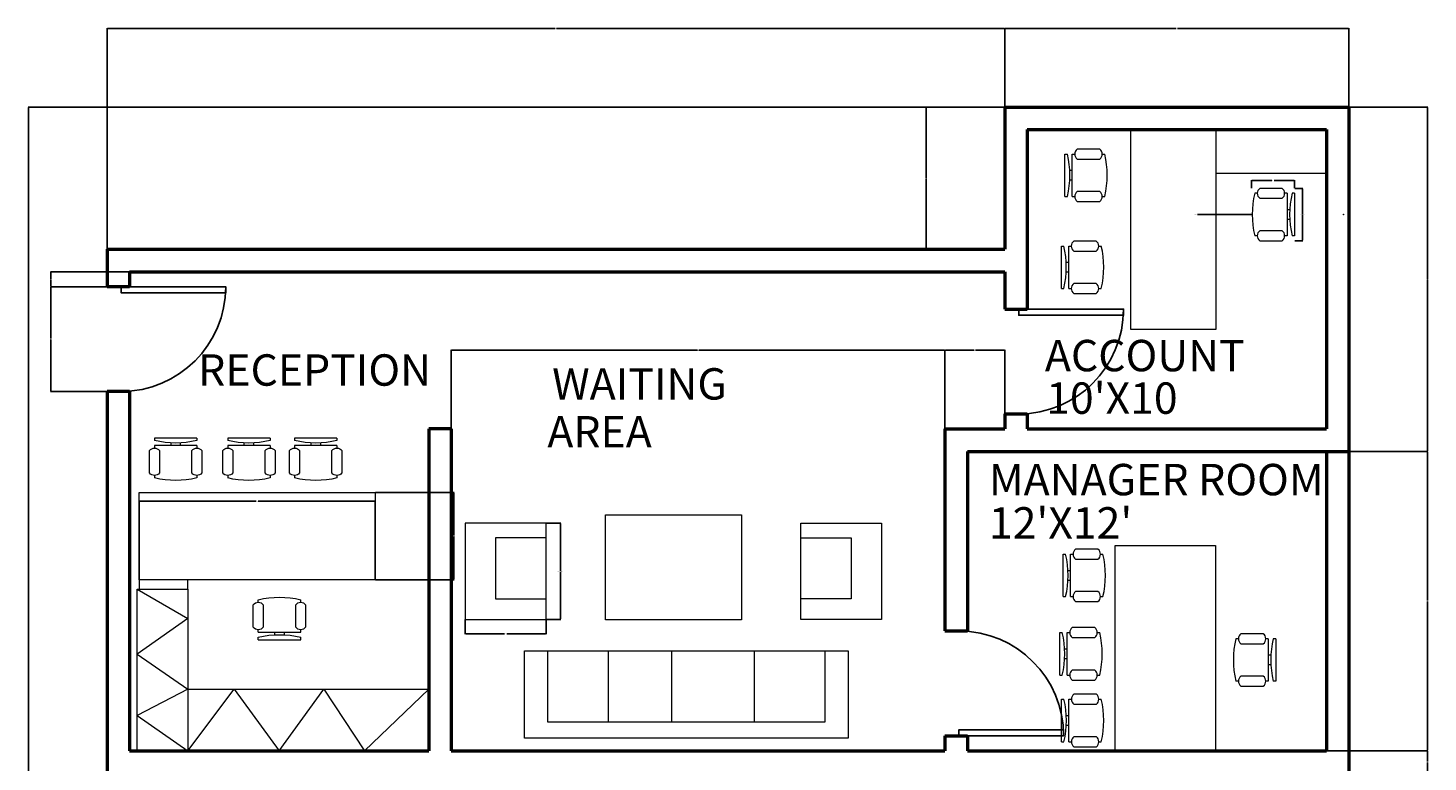
# Model space of a CAD drawing. Units: inches. Extents: x 4242 to 4803, y 4687 to 5377.
# Tile 2 of 2: x 4242 to 4803, y 5083 to 5377. Entities that reach past the tile are written whole.
import ezdxf

# ---------------------------------------------------------------- set-up
doc = ezdxf.new("R2010")
doc.units = ezdxf.units.IN
for name, color, linetype, lineweight in [('A-ANNO-DIMS', 2, 'Continuous', 18), ('A-AREA-IDEN', 7, 'Continuous', 25), ('A-DOOR', 4, 'Continuous', 25), ('A-FURN', 8, 'Continuous', 18), ('A-WALL', 7, 'Continuous', 50)]:
    doc.layers.add(name, color=color, linetype=linetype, lineweight=lineweight)
doc.styles.get("Standard").update_dxf_attribs({"font": 'arial.ttf'})
doc.dimstyles.get("Standard").update_dxf_attribs({"dimtxt": 0.18, "dimasz": 0.18, "dimexe": 0.18, "dimexo": 0.0625, "dimgap": 0.09, "dimtad": 0, "dimtih": 1, "dimtoh": 1, "dimdec": 4, "dimzin": 0, "dimdsep": 46, "dimtxsty": 'Standard', "dimcen": 0.09, "dimadec": 0, "dimazin": 0, "dimtfac": 1, "dimtdec": 4, "dimtofl": 0, "dimtmove": 0, "dimatfit": 3, "dimfxl": 1, "dimtolj": 1, "dimtzin": 0, "dimarcsym": 0})

# ---------------------------------------------------------------- blocks, each defined once
blk = doc.blocks.new('Chair - Desk')
for p, q in [((-8.5, 0), (-8.5, -1)), ((-8.5, 0), (8.5, 0)), ((8.5, 0), (8.5, -1)), ((-10.5, -5), (-10.5, -14)), ((-8.5, -3), (-8.5, -4)), ((-8.5, -3), (8.5, -3)), ((-6.5, -14), (-6.5, -5)), ((-2, -3), (-2, -1.9355)), ((2, -1.9576), (2, -3)), ((6.5, -5), (6.5, -14)), ((8.5, -3), (8.5, -4)), ((10.5, -14), (10.5, -5)), ((-8.5, -15), (-8.5, -16)), ((8.5, -15), (8.5, -16))]:
    blk.add_line(p, q)
for centre, radius, start, end in [((-8.5, -6.5), 2.5, 36.8699, 143.1301), ((0, 34.625), 36.625, 256.5803, 283.4197), ((8.5, -6.5), 2.5, 36.8699, 143.1301), ((-8.5, -12.5), 2.5, 216.8699, 323.1301), ((0, 19.625), 36.625, 256.5803, 283.4197), ((8.5, -12.5), 2.5, 216.8699, 323.1301)]:
    blk.add_arc(centre, radius, start, end)
blk = doc.blocks.new('*U4')
for p, q in [((0, 0), (0, -100)), ((750, 0), (750, -100))]:
    blk.add_line(p, q)
blk.add_lwpolyline([(0, 0), (0, 750), (43.75, 750), (43.75, 0)], close=True)
blk.add_arc((0, 0), 750, 0, 90)
blk = doc.blocks.new('CHAIR-LOUNGE')
for points in [[(32.4, 38.56), (0, 38.56), (0, 0), (32.4, 0)], [(32.4, 32.69), (12.18, 32.69), (12.18, 8.21), (32.4, 8.21)]]:
    blk.add_lwpolyline(points, close=True)
blk = doc.blocks.new('*D6')
at = {"layer": 'A-ANNO-DIMS', "color": 0, "lineweight": -2, "transparency": 16777216}
for p, q in [((4749.57, 5313.06), (4752.84, 5313.06)), ((4752.66, 5312.88), (4752.66, 5302.75)), ((4752.66, 5292.24), (4752.66, 5302.38)), ((4749.57, 5292.06), (4752.84, 5292.06))]:
    blk.add_line(p, q, dxfattribs=at)
at = {"layer": 'A-ANNO-DIMS', "color": 0, "transparency": 16777216}
for points in [[(4752.63, 5312.88), (4752.69, 5312.88), (4752.66, 5313.06)], [(4752.63, 5292.24), (4752.69, 5292.24), (4752.66, 5292.06)]]:
    blk.add_solid(points, dxfattribs=at)
at = {"layer": 'Defpoints', "color": 0, "transparency": 16777216}
for p in [(4749.51, 5313.06), (4749.51, 5292.06), (4752.66, 5292.06)]:
    blk.add_point(p, dxfattribs=at)
at = {"layer": 'A-ANNO-DIMS', "color": 0, "transparency": 16777216, "insert": (4752.66, 5302.56), "char_height": 0.18, "attachment_point": 5}
blk.add_mtext('\\A1;DESK CHAIR 21 TYP.', dxfattribs=at)
blk = doc.blocks.new('*D7')
at = {"layer": 'A-ANNO-DIMS', "color": 0, "lineweight": -2, "transparency": 16777216}
for p, q in [((4732.18, 5313.13), (4732.18, 5316.39)), ((4732.36, 5316.21), (4740.32, 5316.21)), ((4749.33, 5316.21), (4741.36, 5316.21)), ((4749.51, 5313.13), (4749.51, 5316.39))]:
    blk.add_line(p, q, dxfattribs=at)
at = {"layer": 'A-ANNO-DIMS', "color": 0, "transparency": 16777216}
for points in [[(4732.36, 5316.24), (4732.36, 5316.18), (4732.18, 5316.21)], [(4749.33, 5316.24), (4749.33, 5316.18), (4749.51, 5316.21)]]:
    blk.add_solid(points, dxfattribs=at)
at = {"layer": 'Defpoints', "color": 0, "transparency": 16777216}
for p in [(4732.18, 5313.06), (4749.51, 5316.21), (4749.51, 5313.06)]:
    blk.add_point(p, dxfattribs=at)
at = {"layer": 'A-ANNO-DIMS', "color": 0, "transparency": 16777216, "insert": (4740.84, 5316.21), "char_height": 0.18, "attachment_point": 5}
blk.add_mtext('\\A1;17 TYP.', dxfattribs=at)
blk = doc.blocks.new('*D10')
at = {"layer": 'A-ANNO-DIMS', "color": 0, "lineweight": -2, "transparency": 16777216}
for p, q in [((4449.39, 5178.86), (4455.29, 5178.86)), ((4455.11, 5178.68), (4455.11, 5159.77)), ((4455.11, 5140.48), (4455.11, 5159.4)), ((4449.39, 5140.3), (4455.29, 5140.3))]:
    blk.add_line(p, q, dxfattribs=at)
at = {"layer": 'A-ANNO-DIMS', "color": 0, "transparency": 16777216}
for points in [[(4455.08, 5178.68), (4455.14, 5178.68), (4455.11, 5178.86)], [(4455.08, 5140.48), (4455.14, 5140.48), (4455.11, 5140.3)]]:
    blk.add_solid(points, dxfattribs=at)
at = {"layer": 'Defpoints', "color": 0, "transparency": 16777216}
for p in [(4449.33, 5178.86), (4455.11, 5178.86), (4449.33, 5140.3)]:
    blk.add_point(p, dxfattribs=at)
at = {"layer": 'A-ANNO-DIMS', "color": 0, "transparency": 16777216, "insert": (4455.11, 5159.58), "char_height": 0.18, "attachment_point": 5}
blk.add_mtext('\\A1;LOUNGE CHAIR 39 TYP.', dxfattribs=at)
blk = doc.blocks.new('*D11')
at = {"layer": 'A-ANNO-DIMS', "color": 0, "lineweight": -2, "transparency": 16777216}
for p, q in [((4416.93, 5140.24), (4416.93, 5134.34)), ((4449.33, 5140.24), (4449.33, 5134.34)), ((4417.11, 5134.52), (4432.6, 5134.52)), ((4449.15, 5134.52), (4433.65, 5134.52))]:
    blk.add_line(p, q, dxfattribs=at)
at = {"layer": 'A-ANNO-DIMS', "color": 0, "transparency": 16777216}
for points in [[(4417.11, 5134.55), (4417.11, 5134.49), (4416.93, 5134.52)], [(4449.15, 5134.55), (4449.15, 5134.49), (4449.33, 5134.52)]]:
    blk.add_solid(points, dxfattribs=at)
at = {"layer": 'Defpoints', "color": 0, "transparency": 16777216}
for p in [(4416.93, 5140.3), (4449.33, 5140.3), (4449.33, 5134.52)]:
    blk.add_point(p, dxfattribs=at)
at = {"layer": 'A-ANNO-DIMS', "color": 0, "transparency": 16777216, "insert": (4433.13, 5134.52), "char_height": 0.18, "attachment_point": 5}
blk.add_mtext('\\A1;32 TYP.', dxfattribs=at)
blk = doc.blocks.new('*D13')
at = {"layer": 'A-ANNO-DIMS', "color": 0, "lineweight": -2, "transparency": 16777216}
for p, q in [((4633.22, 5345.64), (4241.6, 5345.64)), ((4241.78, 5345.46), (4241.78, 5032.32)), ((4241.78, 4718.82), (4241.78, 5031.96)), ((4273.22, 4718.64), (4241.6, 4718.64))]:
    blk.add_line(p, q, dxfattribs=at)
at = {"layer": 'A-ANNO-DIMS', "color": 0, "transparency": 16777216}
for points in [[(4241.75, 5345.46), (4241.81, 5345.46), (4241.78, 5345.64)], [(4241.75, 4718.82), (4241.81, 4718.82), (4241.78, 4718.64)]]:
    blk.add_solid(points, dxfattribs=at)
at = {"layer": 'Defpoints', "color": 0, "transparency": 16777216}
for p in [(4241.78, 5345.64), (4633.28, 5345.64), (4273.28, 4718.64)]:
    blk.add_point(p, dxfattribs=at)
at = {"layer": 'A-ANNO-DIMS', "color": 0, "transparency": 16777216, "insert": (4241.78, 5032.14), "char_height": 0.18, "attachment_point": 5}
blk.add_mtext('\\A1;627', dxfattribs=at)
blk = doc.blocks.new('*D14')
at = {"layer": 'A-ANNO-DIMS', "color": 0, "lineweight": -2, "transparency": 16777216}
for p, q in [((4273.28, 5288.7), (4273.28, 5377.32)), ((4273.46, 5377.14), (4453, 5377.14)), ((4633.1, 5377.14), (4453.57, 5377.14)), ((4633.28, 5288.7), (4633.28, 5377.32))]:
    blk.add_line(p, q, dxfattribs=at)
at = {"layer": 'A-ANNO-DIMS', "color": 0, "transparency": 16777216}
for points in [[(4273.46, 5377.17), (4273.46, 5377.11), (4273.28, 5377.14)], [(4633.1, 5377.17), (4633.1, 5377.11), (4633.28, 5377.14)]]:
    blk.add_solid(points, dxfattribs=at)
at = {"layer": 'Defpoints', "color": 0, "transparency": 16777216}
for p in [(4633.28, 5377.14), (4273.28, 5288.64), (4633.28, 5288.64)]:
    blk.add_point(p, dxfattribs=at)
at = {"layer": 'A-ANNO-DIMS', "color": 0, "transparency": 16777216, "insert": (4453.28, 5377.14), "char_height": 0.18, "attachment_point": 5}
blk.add_mtext('\\A1;360', dxfattribs=at)
blk = doc.blocks.new('*D15')
at = {"layer": 'A-ANNO-DIMS', "color": 0, "lineweight": -2, "transparency": 16777216}
for p, q in [((4633.28, 5345.7), (4633.28, 5377.32)), ((4633.46, 5377.14), (4702, 5377.14)), ((4771.1, 5377.14), (4702.56, 5377.14)), ((4771.28, 5345.7), (4771.28, 5377.32))]:
    blk.add_line(p, q, dxfattribs=at)
at = {"layer": 'A-ANNO-DIMS', "color": 0, "transparency": 16777216}
for points in [[(4633.46, 5377.17), (4633.46, 5377.11), (4633.28, 5377.14)], [(4771.1, 5377.17), (4771.1, 5377.11), (4771.28, 5377.14)]]:
    blk.add_solid(points, dxfattribs=at)
at = {"layer": 'Defpoints', "color": 0, "transparency": 16777216}
for p in [(4771.28, 5377.14), (4633.28, 5345.64), (4771.28, 5345.64)]:
    blk.add_point(p, dxfattribs=at)
at = {"layer": 'A-ANNO-DIMS', "color": 0, "transparency": 16777216, "insert": (4702.28, 5377.14), "char_height": 0.18, "attachment_point": 5}
blk.add_mtext('\\A1;138', dxfattribs=at)
blk = doc.blocks.new('*D21')
at = {"layer": 'A-ANNO-DIMS', "color": 0, "lineweight": -2, "transparency": 16777216}
for p, q in [((4762.35, 5087.64), (4802.96, 5087.64)), ((4802.78, 5087.46), (4802.78, 5083.32)), ((4802.78, 5078.82), (4802.78, 5082.96)), ((4762.35, 5078.64), (4802.96, 5078.64))]:
    blk.add_line(p, q, dxfattribs=at)
at = {"layer": 'A-ANNO-DIMS', "color": 0, "transparency": 16777216}
for points in [[(4802.75, 5087.46), (4802.81, 5087.46), (4802.78, 5087.64)], [(4802.75, 5078.82), (4802.81, 5078.82), (4802.78, 5078.64)]]:
    blk.add_solid(points, dxfattribs=at)
at = {"layer": 'Defpoints', "color": 0, "transparency": 16777216}
for p in [(4762.28, 5087.64), (4802.78, 5087.64), (4762.28, 5078.64)]:
    blk.add_point(p, dxfattribs=at)
at = {"layer": 'A-ANNO-DIMS', "color": 0, "transparency": 16777216, "insert": (4802.78, 5083.14), "char_height": 0.18, "attachment_point": 5}
blk.add_mtext('\\A1;9', dxfattribs=at)
blk = doc.blocks.new('*D22')
at = {"layer": 'A-ANNO-DIMS', "color": 0, "lineweight": -2, "transparency": 16777216}
for p, q in [((4762.35, 5207.64), (4802.96, 5207.64)), ((4802.78, 5207.46), (4802.78, 5147.82)), ((4802.78, 5087.82), (4802.78, 5147.46)), ((4762.35, 5087.64), (4802.96, 5087.64))]:
    blk.add_line(p, q, dxfattribs=at)
at = {"layer": 'A-ANNO-DIMS', "color": 0, "transparency": 16777216}
for points in [[(4802.75, 5207.46), (4802.81, 5207.46), (4802.78, 5207.64)], [(4802.75, 5087.82), (4802.81, 5087.82), (4802.78, 5087.64)]]:
    blk.add_solid(points, dxfattribs=at)
at = {"layer": 'Defpoints', "color": 0, "transparency": 16777216}
for p in [(4762.28, 5207.64), (4802.78, 5207.64), (4762.28, 5087.64)]:
    blk.add_point(p, dxfattribs=at)
at = {"layer": 'A-ANNO-DIMS', "color": 0, "transparency": 16777216, "insert": (4802.78, 5147.64), "char_height": 0.18, "attachment_point": 5}
blk.add_mtext('\\A1;120', dxfattribs=at)
blk = doc.blocks.new('*D23')
at = {"layer": 'A-ANNO-DIMS', "color": 0, "lineweight": -2, "transparency": 16777216}
for p, q in [((4771.35, 5345.64), (4802.96, 5345.64)), ((4802.78, 5345.46), (4802.78, 5276.82)), ((4802.78, 5207.82), (4802.78, 5276.46)), ((4762.35, 5207.64), (4802.96, 5207.64))]:
    blk.add_line(p, q, dxfattribs=at)
at = {"layer": 'A-ANNO-DIMS', "color": 0, "transparency": 16777216}
for points in [[(4802.75, 5345.46), (4802.81, 5345.46), (4802.78, 5345.64)], [(4802.75, 5207.82), (4802.81, 5207.82), (4802.78, 5207.64)]]:
    blk.add_solid(points, dxfattribs=at)
at = {"layer": 'Defpoints', "color": 0, "transparency": 16777216}
for p in [(4771.28, 5345.64), (4802.78, 5345.64), (4762.28, 5207.64)]:
    blk.add_point(p, dxfattribs=at)
at = {"layer": 'A-ANNO-DIMS', "color": 0, "transparency": 16777216, "insert": (4802.78, 5276.64), "char_height": 0.18, "attachment_point": 5}
blk.add_mtext('\\A1;138', dxfattribs=at)
blk = doc.blocks.new('*D24')
at = {"layer": 'A-ANNO-DIMS', "color": 0, "lineweight": -2, "transparency": 16777216}
for p, q in [((4633.22, 5345.64), (4601.6, 5345.64)), ((4601.78, 5345.46), (4601.78, 5317.32)), ((4601.78, 5288.82), (4601.78, 5316.96)), ((4633.22, 5288.64), (4601.6, 5288.64))]:
    blk.add_line(p, q, dxfattribs=at)
at = {"layer": 'A-ANNO-DIMS', "color": 0, "transparency": 16777216}
for points in [[(4601.75, 5345.46), (4601.81, 5345.46), (4601.78, 5345.64)], [(4601.75, 5288.82), (4601.81, 5288.82), (4601.78, 5288.64)]]:
    blk.add_solid(points, dxfattribs=at)
at = {"layer": 'Defpoints', "color": 0, "transparency": 16777216}
for p in [(4601.78, 5345.64), (4633.28, 5345.64), (4633.28, 5288.64)]:
    blk.add_point(p, dxfattribs=at)
at = {"layer": 'A-ANNO-DIMS', "color": 0, "transparency": 16777216, "insert": (4601.78, 5317.14), "char_height": 0.18, "attachment_point": 5}
blk.add_mtext('\\A1;57', dxfattribs=at)
blk = doc.blocks.new('*D26')
at = {"layer": 'A-ANNO-DIMS', "color": 0, "lineweight": -2, "transparency": 16777216}
for p, q in [((4282.22, 5273.64), (4250.6, 5273.64)), ((4250.78, 5273.46), (4250.78, 5252.82)), ((4250.78, 5231.82), (4250.78, 5252.46)), ((4282.22, 5231.64), (4250.6, 5231.64))]:
    blk.add_line(p, q, dxfattribs=at)
at = {"layer": 'A-ANNO-DIMS', "color": 0, "transparency": 16777216}
for points in [[(4250.75, 5273.46), (4250.81, 5273.46), (4250.78, 5273.64)], [(4250.75, 5231.82), (4250.81, 5231.82), (4250.78, 5231.64)]]:
    blk.add_solid(points, dxfattribs=at)
at = {"layer": 'Defpoints', "color": 0, "transparency": 16777216}
for p in [(4250.78, 5273.64), (4282.28, 5273.64), (4282.28, 5231.64)]:
    blk.add_point(p, dxfattribs=at)
at = {"layer": 'A-ANNO-DIMS', "color": 0, "transparency": 16777216, "insert": (4250.78, 5252.64), "char_height": 0.18, "attachment_point": 5}
blk.add_mtext('\\A1;42', dxfattribs=at)
blk = doc.blocks.new('*D27')
at = {"layer": 'A-ANNO-DIMS', "color": 0, "lineweight": -2, "transparency": 16777216}
for p, q in [((4282.22, 5279.64), (4250.6, 5279.64)), ((4250.78, 5279.46), (4250.78, 5276.82)), ((4282.22, 5273.64), (4250.6, 5273.64)), ((4250.78, 5273.82), (4250.78, 5276.46))]:
    blk.add_line(p, q, dxfattribs=at)
at = {"layer": 'A-ANNO-DIMS', "color": 0, "transparency": 16777216}
for points in [[(4250.75, 5279.46), (4250.81, 5279.46), (4250.78, 5279.64)], [(4250.75, 5273.82), (4250.81, 5273.82), (4250.78, 5273.64)]]:
    blk.add_solid(points, dxfattribs=at)
at = {"layer": 'Defpoints', "color": 0, "transparency": 16777216}
for p in [(4250.78, 5279.64), (4282.28, 5279.64), (4282.28, 5273.64)]:
    blk.add_point(p, dxfattribs=at)
at = {"layer": 'A-ANNO-DIMS', "color": 0, "transparency": 16777216, "insert": (4250.78, 5276.64), "char_height": 0.18, "attachment_point": 5}
blk.add_mtext('\\A1;6', dxfattribs=at)
blk = doc.blocks.new('*D30')
at = {"layer": 'A-ANNO-DIMS', "color": 0, "lineweight": -2, "transparency": 16777216}
for p, q in [((4411.28, 5216.7), (4411.28, 5248.32)), ((4411.46, 5248.14), (4510, 5248.14)), ((4609.1, 5248.14), (4510.56, 5248.14)), ((4609.28, 5216.7), (4609.28, 5248.32))]:
    blk.add_line(p, q, dxfattribs=at)
at = {"layer": 'A-ANNO-DIMS', "color": 0, "transparency": 16777216}
for points in [[(4411.46, 5248.17), (4411.46, 5248.11), (4411.28, 5248.14)], [(4609.1, 5248.17), (4609.1, 5248.11), (4609.28, 5248.14)]]:
    blk.add_solid(points, dxfattribs=at)
at = {"layer": 'Defpoints', "color": 0, "transparency": 16777216}
for p in [(4609.28, 5248.14), (4411.28, 5216.64), (4609.28, 5216.64)]:
    blk.add_point(p, dxfattribs=at)
at = {"layer": 'A-ANNO-DIMS', "color": 0, "transparency": 16777216, "insert": (4510.28, 5248.14), "char_height": 0.18, "attachment_point": 5}
blk.add_mtext('\\A1;198', dxfattribs=at)
blk = doc.blocks.new('*D31')
at = {"layer": 'A-ANNO-DIMS', "color": 0, "lineweight": -2, "transparency": 16777216}
for p, q in [((4609.28, 5216.7), (4609.28, 5248.32)), ((4609.46, 5248.14), (4621.06, 5248.14)), ((4633.1, 5248.14), (4621.5, 5248.14)), ((4633.28, 5216.7), (4633.28, 5248.32))]:
    blk.add_line(p, q, dxfattribs=at)
at = {"layer": 'A-ANNO-DIMS', "color": 0, "transparency": 16777216}
for points in [[(4609.46, 5248.17), (4609.46, 5248.11), (4609.28, 5248.14)], [(4633.1, 5248.17), (4633.1, 5248.11), (4633.28, 5248.14)]]:
    blk.add_solid(points, dxfattribs=at)
at = {"layer": 'Defpoints', "color": 0, "transparency": 16777216}
for p in [(4633.28, 5248.14), (4609.28, 5216.64), (4633.28, 5216.64)]:
    blk.add_point(p, dxfattribs=at)
at = {"layer": 'A-ANNO-DIMS', "color": 0, "transparency": 16777216, "insert": (4621.28, 5248.14), "char_height": 0.18, "attachment_point": 5}
blk.add_mtext('\\A1;24', dxfattribs=at)
blk = doc.blocks.new('*D37')
at = {"layer": 'A-ANNO-DIMS', "color": 0, "lineweight": -2, "transparency": 16777216}
for p, q in [((4286.13, 5156.26), (4286.13, 5187.88)), ((4286.31, 5187.7), (4333.08, 5187.7)), ((4380.64, 5187.7), (4333.87, 5187.7)), ((4380.82, 5156.26), (4380.82, 5187.88))]:
    blk.add_line(p, q, dxfattribs=at)
at = {"layer": 'A-ANNO-DIMS', "color": 0, "transparency": 16777216}
for points in [[(4286.31, 5187.73), (4286.31, 5187.67), (4286.13, 5187.7)], [(4380.64, 5187.73), (4380.64, 5187.67), (4380.82, 5187.7)]]:
    blk.add_solid(points, dxfattribs=at)
at = {"layer": 'Defpoints', "color": 0, "transparency": 16777216}
for p in [(4380.82, 5187.7), (4286.13, 5156.2), (4380.82, 5156.2)]:
    blk.add_point(p, dxfattribs=at)
at = {"layer": 'A-ANNO-DIMS', "color": 0, "transparency": 16777216, "insert": (4333.47, 5187.7), "char_height": 0.18, "attachment_point": 5}
blk.add_mtext('\\A1;94.69', dxfattribs=at)
blk = doc.blocks.new('*D38')
at = {"layer": 'A-ANNO-DIMS', "color": 0, "lineweight": -2, "transparency": 16777216}
for p, q in [((4380.88, 5191.18), (4412.5, 5191.18)), ((4412.32, 5191), (4412.32, 5173.87)), ((4412.32, 5156.38), (4412.32, 5173.51)), ((4380.88, 5156.2), (4412.5, 5156.2))]:
    blk.add_line(p, q, dxfattribs=at)
at = {"layer": 'A-ANNO-DIMS', "color": 0, "transparency": 16777216}
for points in [[(4412.29, 5191), (4412.35, 5191), (4412.32, 5191.18)], [(4412.29, 5156.38), (4412.35, 5156.38), (4412.32, 5156.2)]]:
    blk.add_solid(points, dxfattribs=at)
at = {"layer": 'Defpoints', "color": 0, "transparency": 16777216}
for p in [(4380.82, 5191.18), (4380.82, 5156.2), (4412.32, 5156.2)]:
    blk.add_point(p, dxfattribs=at)
at = {"layer": 'A-ANNO-DIMS', "color": 0, "transparency": 16777216, "insert": (4412.32, 5173.69), "char_height": 0.18, "attachment_point": 5}
blk.add_mtext('\\A1;34.98', dxfattribs=at)
blk = doc.blocks.new('*D41')
at = {"layer": 'A-ANNO-DIMS', "color": 0, "lineweight": -2, "transparency": 16777216}
for p, q in [((4710.54, 5302.56), (4732.33, 5302.56)), ((4769.05, 5302.56), (4769.23, 5302.56)), ((4769.14, 5302.47), (4769.14, 5302.65))]:
    blk.add_line(p, q, dxfattribs=at)
at = {"layer": 'A-ANNO-DIMS', "color": 0, "transparency": 16777216}
blk.add_solid([(4732.33, 5302.59), (4732.33, 5302.53), (4732.51, 5302.56)], dxfattribs=at)
at = {"layer": 'Defpoints', "color": 0, "transparency": 16777216}
for p in [(4732.51, 5302.56), (4769.14, 5302.56)]:
    blk.add_point(p, dxfattribs=at)
at = {"layer": 'A-ANNO-DIMS', "color": 0, "transparency": 16777216, "insert": (4709.72, 5302.56), "char_height": 0.18, "attachment_point": 5}
blk.add_mtext('\\A1;25X R36.625', dxfattribs=at)

msp = doc.modelspace()

# ---------------------------------------------------------------- linework, layer by layer
at = {"layer": 'A-FURN'}
for p, q in [((4305.7309, 5156.1997), (4286.1298, 5156.1997)), ((4286.1298, 5156.1997), (4286.1298, 5152.4595)), ((4305.7309, 5152.4595), (4305.7309, 5156.1997)), ((4285.3425, 5152.4595), (4305.7309, 5140.6038)), ((4305.7309, 5140.6038), (4285.3425, 5126.3034)), ((4285.3425, 5126.3034), (4305.7309, 5112.3436)), ((4474.2273, 5127.7417), (4474.2273, 5099.1557)), ((4499.6923, 5127.7417), (4499.6923, 5099.1557)), ((4532.7665, 5127.7417), (4532.7665, 5099.1557)), ((4305.7309, 5112.3436), (4285.3425, 5101.7886)), ((4305.7309, 5112.3436), (4402.2844, 5112.3436)), ((4305.7309, 5087.6424), (4324.2313, 5112.3436)), ((4324.2313, 5112.3436), (4342.2844, 5087.6424)), ((4342.2844, 5087.6424), (4360.2218, 5112.3436)), ((4360.2218, 5112.3436), (4376.5813, 5087.6424)), ((4376.5813, 5087.6424), (4402.2844, 5112.3436)), ((4285.3425, 5101.7886), (4305.7309, 5087.6424))]:
    msp.add_line(p, q, dxfattribs=at)
for points in [[(4683.8095, 5336.6424), (4717.8618, 5336.6424), (4717.8618, 5256.4191), (4683.8095, 5256.4191)], [(4717.8618, 5319.1468), (4762.2844, 5319.1468), (4762.2844, 5336.6424), (4717.8618, 5336.6424)], [(4286.1298, 5191.1814), (4380.8184, 5191.1814), (4380.8184, 5156.1997), (4286.1298, 5156.1997)], [(4473.1461, 5182.2525), (4527.6766, 5182.2525), (4527.6766, 5140.0874), (4473.1461, 5140.0874)], [(4677.506, 5169.9646), (4717.7432, 5169.9646), (4717.7432, 5087.6424), (4677.506, 5087.6424)], [(4285.3425, 5152.4595), (4305.7309, 5152.4595), (4305.7309, 5087.6424), (4285.3425, 5087.6424)], [(4440.6947, 5127.7417), (4570.4138, 5127.7417), (4570.4138, 5092.6338), (4440.6947, 5092.6338)], [(4450.0905, 5127.7417), (4561.0505, 5127.7417), (4561.0505, 5099.1557), (4450.0905, 5099.1557)]]:
    msp.add_lwpolyline(points, close=True, dxfattribs=at)
at = {"layer": 'A-WALL'}
for p, q in [((4633.2844, 5345.6424), (4633.2844, 5288.6424)), ((4633.2844, 5345.6424), (4771.2844, 5345.6424)), ((4771.2844, 5345.6424), (4771.2844, 5009.6424)), ((4642.2844, 5336.6424), (4642.2844, 5264.6424)), ((4642.2844, 5336.6424), (4762.2844, 5336.6424)), ((4762.2844, 5336.6424), (4762.2844, 5216.6424)), ((4273.2844, 5288.6424), (4633.2844, 5288.6424)), ((4273.2844, 5288.6424), (4273.2844, 5273.6424)), ((4282.2844, 5279.6424), (4633.2844, 5279.6424)), ((4282.2844, 5279.6424), (4282.2844, 5273.6424)), ((4633.2844, 5279.6424), (4633.2844, 5264.6424)), ((4282.2844, 5273.6424), (4273.2844, 5273.6424)), ((4633.2844, 5264.6424), (4642.2844, 5264.6424)), ((4282.2844, 5231.6424), (4273.2844, 5231.6424)), ((4273.2844, 5231.6424), (4273.2844, 4718.6424)), ((4282.2844, 5231.6424), (4282.2844, 5087.6424)), ((4633.2844, 5222.6424), (4642.2844, 5222.6424)), ((4633.2844, 5222.6424), (4633.2844, 5216.6424)), ((4642.2844, 5222.6424), (4642.2844, 5216.6424)), ((4402.2844, 5216.6424), (4402.2844, 5087.6424)), ((4411.2844, 5216.6424), (4402.2844, 5216.6424)), ((4411.2844, 5216.6424), (4411.2844, 5087.6424)), ((4609.2844, 5216.6424), (4633.2844, 5216.6424)), ((4609.2844, 5216.6424), (4609.2844, 5135.6424)), ((4642.2844, 5216.6424), (4762.2844, 5216.6424)), ((4618.2844, 5207.6424), (4771.2844, 5207.6424)), ((4618.2844, 5207.6424), (4618.2844, 5135.6424)), ((4762.2844, 5207.6424), (4762.2844, 5087.6424)), ((4609.2844, 5135.6424), (4618.2844, 5135.6424)), ((4609.2844, 5093.6424), (4618.2844, 5093.6424)), ((4609.2844, 5093.6424), (4609.2844, 5087.6424)), ((4618.2844, 5093.6424), (4618.2844, 5087.6424)), ((4282.2844, 5087.6424), (4402.2844, 5087.6424)), ((4411.2844, 5087.6424), (4609.2844, 5087.6424)), ((4618.2844, 5087.6424), (4633.2844, 5087.6424)), ((4633.2844, 5087.6424), (4762.2844, 5087.6424))]:
    msp.add_line(p, q, dxfattribs=at)

# ---------------------------------------------------------------- block references
at = {"layer": 'A-DOOR', "yscale": 0.0559999999999998, "zscale": 0.0559999999999998, "rotation": 270}
for p, xscale in [((4278.8844, 5273.6424), 0.0559999999999998), ((4638.8844, 5264.6424), 0.0559999999999998), ((4614.8844, 5093.6424), -0.0559999999999998)]:
    msp.add_blockref('*U4', p, dxfattribs=dict(at, xscale=xscale))
at = {"layer": 'A-FURN'}
for p, rotation in [((4657.3632, 5318.2826), 90), ((4749.5106, 5302.5627), 270), ((4655.9576, 5281.4314), 90), ((4656.6552, 5157.9143), 90), ((4655.327, 5126.497), 90), ((4741.9397, 5124.044), 270), ((4655.9906, 5099.7653), 90)]:
    msp.add_blockref('Chair - Desk', p, dxfattribs=dict(at, rotation=rotation))
at = {"layer": 'A-FURN', "xscale": -1}
for p in [(4300.7963, 5212.9768), (4330.1754, 5212.9768), (4356.9838, 5212.9768)]:
    msp.add_blockref('Chair - Desk', p, dxfattribs=at)
at = {"layer": 'A-FURN'}
msp.add_blockref('CHAIR-LOUNGE', (4416.9261, 5140.3041), dxfattribs=at)
at = {"layer": 'A-FURN', "extrusion": (0, 0, -1), "zscale": -1}
msp.add_blockref('CHAIR-LOUNGE', (-4583.8967, 5140.3041), dxfattribs=at)
at = {"layer": 'A-FURN', "xscale": -1, "rotation": 180}
msp.add_blockref('Chair - Desk', (4342.4219, 5132.1673), dxfattribs=at)

# ---------------------------------------------------------------- texts
at = {"layer": 'A-AREA-IDEN'}
for s, p in [('ACCOUNT', (4649.3675, 5239.7453)), ('RECEPTION', (4309.815, 5233.9539)), ('WAITING', (4451.7574, 5228.3982)), ("10'X10", (4649.8697, 5222.6921)), ('AREA', (4449.8352, 5209.2006)), ('MANAGER ROOM', (4626.9054, 5190.0395)), ("12'X12'", (4626.9054, 5172.6876))]:
    msp.add_text(s, height=12.5832, dxfattribs=at).set_placement(p)

# ---------------------------------------------------------------- dimensions: what is measured, and where the dimension line sits
at = {"layer": 'A-ANNO-DIMS'}
for base, p1, p2, override, picture, middle in [((4633.2844, 5377.1424), (4273.2844, 5288.6424), (4633.2844, 5288.6424), {"dimdec": 0, "dimlfac": 1, "dimrnd": 0, "dimzin": 0, "dimdsep": 46, "dimlunit": 2}, '*D14', (4453.2844, 5377.1424)), ((4771.2844, 5377.1424), (4633.2844, 5345.6424), (4771.2844, 5345.6424), {"dimdec": 0, "dimlfac": 1, "dimrnd": 0, "dimzin": 0, "dimdsep": 46, "dimlunit": 2}, '*D15', (4702.2844, 5377.1424)), ((4609.2844, 5248.1424), (4411.2844, 5216.6424), (4609.2844, 5216.6424), {"dimdec": 0, "dimlfac": 1, "dimrnd": 0, "dimzin": 0, "dimdsep": 46, "dimlunit": 2}, '*D30', (4510.2844, 5248.1424)), ((4633.2844, 5248.1424), (4609.2844, 5216.6424), (4633.2844, 5216.6424), {"dimdec": 0, "dimlfac": 1, "dimrnd": 0, "dimzin": 0, "dimdsep": 46, "dimlunit": 2}, '*D31', (4621.2844, 5248.1424)), ((4380.8184, 5187.6997), (4286.1298, 5156.1997), (4380.8184, 5156.1997), {"dimdec": 2, "dimlfac": 1, "dimrnd": 0, "dimzin": 0, "dimdsep": 46, "dimlunit": 2}, '*D37', (4333.4741, 5187.6997))]:
    dim = msp.add_linear_dim(base=base, p1=p1, p2=p2, dimstyle='Standard', override=override, dxfattribs=at)
    dim.commit()
    dim.dimension.update_dxf_attribs({"geometry": picture, "text_midpoint": middle})
for base, p1, p2, angle, override, picture, middle in [((4241.7844, 5345.6424), (4273.2844, 4718.6424), (4633.2844, 5345.6424), 90, {"dimdec": 0, "dimlfac": 1, "dimrnd": 0, "dimzin": 0, "dimdsep": 46, "dimlunit": 2}, '*D13', (4241.7844, 5032.1424)), ((4601.7844, 5345.6424), (4633.2844, 5288.6424), (4633.2844, 5345.6424), 90, {"dimdec": 0, "dimlfac": 1, "dimrnd": 0, "dimzin": 0, "dimdsep": 46, "dimlunit": 2}, '*D24', (4601.7844, 5317.1424)), ((4802.7844, 5345.6424), (4762.2844, 5207.6424), (4771.2844, 5345.6424), 90, {"dimdec": 0, "dimlfac": 1, "dimrnd": 0, "dimzin": 0, "dimdsep": 46, "dimlunit": 2}, '*D23', (4802.7844, 5276.6424)), ((4250.7844, 5279.6424), (4282.2844, 5273.6424), (4282.2844, 5279.6424), 90, {"dimdec": 0, "dimlfac": 1, "dimrnd": 0, "dimzin": 0, "dimdsep": 46, "dimlunit": 2}, '*D27', (4250.7844, 5276.6424)), ((4250.7844, 5273.6424), (4282.2844, 5231.6424), (4282.2844, 5273.6424), 90, {"dimdec": 0, "dimlfac": 1, "dimrnd": 0, "dimzin": 0, "dimdsep": 46, "dimlunit": 2}, '*D26', (4250.7844, 5252.6424)), ((4802.7844, 5207.6424), (4762.2844, 5087.6424), (4762.2844, 5207.6424), 90, {"dimdec": 0, "dimlfac": 1, "dimrnd": 0, "dimzin": 0, "dimdsep": 46, "dimlunit": 2}, '*D22', (4802.7844, 5147.6424)), ((4412.3184, 5156.1997), (4380.8184, 5191.1814), (4380.8184, 5156.1997), 270, {"dimdec": 2, "dimlfac": 1, "dimrnd": 0, "dimzin": 0, "dimdsep": 46, "dimlunit": 2}, '*D38', (4412.3184, 5173.6905)), ((4802.7844, 5087.6424), (4762.2844, 5078.6424), (4762.2844, 5087.6424), 90, {"dimdec": 0, "dimlfac": 1, "dimrnd": 0, "dimzin": 0, "dimdsep": 46, "dimlunit": 2}, '*D21', (4802.7844, 5083.1424))]:
    dim = msp.add_linear_dim(base=base, p1=p1, p2=p2, angle=angle, dimstyle='Standard', override=override, dxfattribs=at)
    dim.commit()
    dim.dimension.update_dxf_attribs({"geometry": picture, "text_midpoint": middle})
for base, p1, p2, picture, middle in [((4749.5106, 5316.2127), (4732.1773, 5313.0627), (4749.5106, 5313.0627), '*D7', (4740.8439, 5316.2127)), ((4449.3262, 5134.5205), (4416.9261, 5140.3041), (4449.3262, 5140.3041), '*D11', (4433.1261, 5134.5205))]:
    dim = msp.add_linear_dim(base=base, p1=p1, p2=p2, text='<> TYP.', dimstyle='Standard', override={"dimdec": 0, "dimlfac": 1, "dimrnd": 0, "dimzin": 0, "dimdsep": 46, "dimlunit": 2}, dxfattribs=at)
    dim.commit()
    dim.dimension.update_dxf_attribs({"geometry": picture, "text_midpoint": middle})
for base, p1, p2, angle, text, picture, middle in [((4752.6606, 5292.0627), (4749.5106, 5313.0627), (4749.5106, 5292.0627), 270, 'DESK CHAIR <> TYP.', '*D6', (4752.6606, 5302.5627)), ((4455.1098, 5178.861), (4449.3262, 5140.3041), (4449.3262, 5178.861), 90, 'LOUNGE CHAIR <> TYP.', '*D10', (4455.1098, 5159.5825))]:
    dim = msp.add_linear_dim(base=base, p1=p1, p2=p2, angle=angle, text=text, dimstyle='Standard', override={"dimdec": 0, "dimlfac": 1, "dimrnd": 0, "dimzin": 0, "dimdsep": 46, "dimlunit": 2}, dxfattribs=at)
    dim.commit()
    dim.dimension.update_dxf_attribs({"geometry": picture, "text_midpoint": middle})
dim = msp.add_radius_dim(center=(4769.1356, 5302.5627), mpoint=(4732.5106, 5302.563), text='25X <>', dimstyle='Standard', override={"dimdec": 3, "dimlfac": 1, "dimrnd": 0, "dimzin": 0, "dimdsep": 46, "dimlunit": 2}, dxfattribs=at)
dim.commit()
dim.dimension.update_dxf_attribs({"geometry": '*D41', "text_midpoint": (4710.5356, 5302.5632), "dimtype": 164})

doc.saveas('drawing.dxf')
